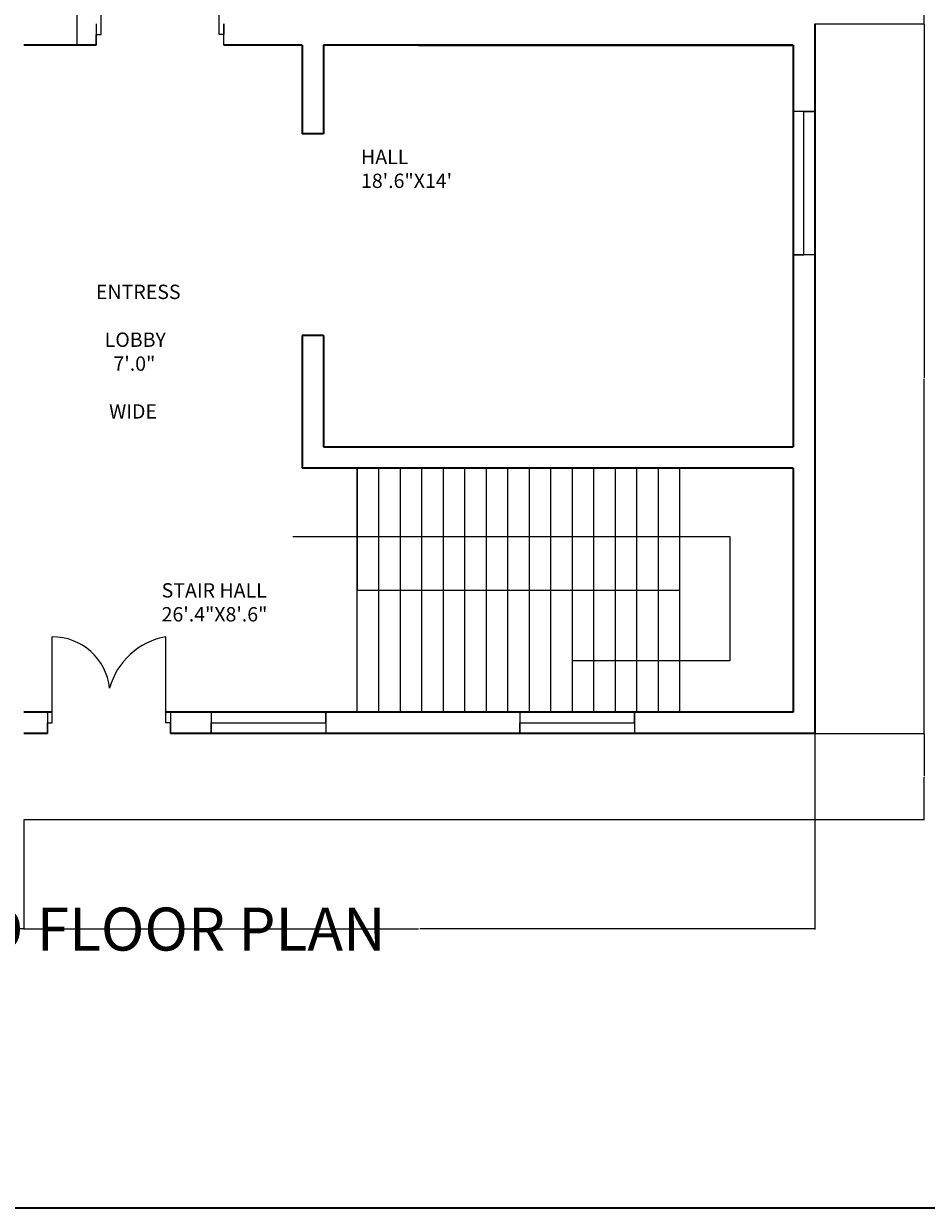
# Model space of a CAD drawing. Units: inches. Extents: x 1824 to 3509, y 619 to 2294.
# Tile 2 of 12: x 2192 to 2570, y 619 to 1115. Entities that reach past the tile are written whole.
import ezdxf

# ---------------------------------------------------------------- set-up
doc = ezdxf.new("R2010")
doc.units = ezdxf.units.IN
for name, color, linetype, lineweight in [('A-ANNO-DIMS', 2, 'Continuous', 18), ('A-ANNO-TEXT', 7, 'Continuous', 25), ('A-ANNO-TTLB', 7, 'Continuous', 35), ('A-AREA-IDEN', 7, 'Continuous', 18), ('A-DOOR', 3, 'Continuous', 18), ('A-FLOR-STRS', 7, 'Continuous', 18), ('A-GLAZ', 4, 'Continuous', 18), ('A-WALL', 7, 'Continuous', 35)]:
    doc.layers.add(name, color=color, linetype=linetype, lineweight=lineweight)
doc.styles.get("Standard").update_dxf_attribs({"font": 'arial.ttf'})
doc.dimstyles.get("Standard").update_dxf_attribs({"dimtxt": 0.18, "dimasz": 0.18, "dimexe": 0.18, "dimexo": 0.0625, "dimgap": 0.09, "dimtad": 0, "dimtih": 1, "dimtoh": 1, "dimdec": 4, "dimzin": 0, "dimdsep": 46, "dimtxsty": 'Standard', "dimcen": 0.09, "dimadec": 0, "dimazin": 0, "dimtfac": 1, "dimtdec": 4, "dimtofl": 0, "dimtmove": 0, "dimatfit": 3, "dimfxl": 1, "dimtolj": 1, "dimtzin": 0, "dimarcsym": 0})

# ---------------------------------------------------------------- blocks, each defined once
blk = doc.blocks.new('STAIR-RETURN-PLAN')
for p, q in [((26.85, 0), (26.85, 102)), ((26.85, 102), (26.85, 51)), ((35.85, 102), (35.85, 0)), ((44.85, 102), (44.85, 0)), ((53.85, 102), (53.85, 0)), ((62.85, 102), (62.85, 0)), ((71.85, 102), (71.85, 0)), ((80.85, 102), (80.85, 0)), ((89.85, 102), (89.85, 0)), ((98.85, 102), (98.85, 0)), ((107.85, 102), (107.85, 0)), ((116.85, 102), (116.85, 0)), ((125.85, 102), (125.85, 0)), ((134.85, 102), (134.85, 0)), ((143.85, 102), (143.85, 0)), ((152.85, 102), (152.85, 0)), ((161.85, 102), (161.85, 0)), ((0, 73.44), (182.85, 73.44)), ((182.85, 73.44), (182.85, 21.48)), ((26.85, 51), (161.85, 51)), ((182.85, 21.48), (116.85, 21.48))]:
    blk.add_line(p, q)
blk = doc.blocks.new('DOOR-LOUNGE-PAIR')
for p, q in [((2, 4.5), (2, 40.5)), ((51.41, 4.5), (51.41, 40.5)), ((27.9, 14.63), (27.9, 18.05)), ((0, 9), (0, 0)), ((53.41, 0), (53.41, 9)), ((53.41, 9), (53.41, 4.5)), ((0, 0), (0, 4.5)), ((0, 4.5), (2, 4.5)), ((53.41, 4.5), (51.41, 4.5)), ((53.41, 4.5), (53.41, 4.5))]:
    blk.add_line(p, q)
for centre, radius, start, end in [((-0.78, 11.81), 28.82, 5.6014, 84.4566), ((54.5, 13.67), 27.01, 96.5732, 173.8895)]:
    blk.add_arc(centre, radius, start, end)
blk = doc.blocks.new('DOOR-ENTRY-PAIR')
for p, q in [((2, 4.5), (2, 40.5)), ((49.54, 4.5), (49.54, 40.5)), ((0, 9), (0, 0)), ((51.54, 9), (51.54, 0)), ((0, 0), (0, 4.5)), ((0, 4.5), (2, 4.5)), ((51.54, 4.5), (49.54, 4.5)), ((51.54, 0), (51.54, 4.5))]:
    blk.add_line(p, q)
for centre, radius, start, end in [((2, 16.28), 24.22, 6.4131, 90), ((54.84, 11.16), 29.82, 100.2425, 164.7797)]:
    blk.add_arc(centre, radius, start, end)
blk = doc.blocks.new('WIN-48')
for p, q in [((0, 9), (0, 0)), ((48, 4.5), (48, 9)), ((48, 9), (48, 0)), ((0, 0), (0, 4.5)), ((0, 4.5), (48, 4.5))]:
    blk.add_line(p, q)
blk = doc.blocks.new('WIN-60')
for p, q in [((0, 9), (0, 0)), ((60, 4.5), (60, 9)), ((60, 9), (60, 0)), ((0, 0), (0, 4.5)), ((0, 4.5), (60, 4.5))]:
    blk.add_line(p, q)
blk = doc.blocks.new('*D75')
at = {"layer": 'A-ANNO-DIMS', "color": 0, "lineweight": -2, "transparency": 16777216}
for p, q in [((2222.38, 1146.6), (2214.25, 1146.6)), ((2214.43, 1146.42), (2214.43, 1126.53)), ((2214.43, 1106.28), (2214.43, 1126.17)), ((2222.38, 1106.1), (2214.25, 1106.1))]:
    blk.add_line(p, q, dxfattribs=at)
at = {"layer": 'A-ANNO-DIMS', "color": 0, "transparency": 16777216}
for points in [[(2214.4, 1146.42), (2214.46, 1146.42), (2214.43, 1146.6)], [(2214.4, 1106.28), (2214.46, 1106.28), (2214.43, 1106.1)]]:
    blk.add_solid(points, dxfattribs=at)
at = {"layer": 'Defpoints', "color": 0, "transparency": 16777216}
for p in [(2214.43, 1146.6), (2222.44, 1146.6), (2222.44, 1106.1)]:
    blk.add_point(p, dxfattribs=at)
at = {"layer": 'A-ANNO-DIMS', "color": 0, "transparency": 16777216, "insert": (2214.43, 1126.35), "char_height": 0.18, "attachment_point": 5}
blk.add_mtext('\\A1;41 TYP.', dxfattribs=at)
blk = doc.blocks.new('*D94')
at = {"layer": 'A-ANNO-DIMS', "color": 0, "lineweight": -2, "transparency": 16777216}
for p, q in [((1949.09, 1049.16), (1949.09, 1668.03)), ((1949.27, 1667.85), (2235.8, 1667.85)), ((2522.91, 1667.85), (2236.38, 1667.85)), ((2523.09, 1622.16), (2523.09, 1668.03))]:
    blk.add_line(p, q, dxfattribs=at)
at = {"layer": 'A-ANNO-DIMS', "color": 0, "transparency": 16777216}
for points in [[(1949.27, 1667.88), (1949.27, 1667.82), (1949.09, 1667.85)], [(2522.91, 1667.88), (2522.91, 1667.82), (2523.09, 1667.85)]]:
    blk.add_solid(points, dxfattribs=at)
at = {"layer": 'Defpoints', "color": 0, "transparency": 16777216}
for p in [(2523.09, 1667.85), (2523.09, 1622.1), (1949.09, 1049.1)]:
    blk.add_point(p, dxfattribs=at)
at = {"layer": 'A-ANNO-DIMS', "color": 0, "transparency": 16777216, "insert": (2236.09, 1667.85), "char_height": 0.18, "attachment_point": 5}
blk.add_mtext('\\A1;574', dxfattribs=at)
blk = doc.blocks.new('*D96')
at = {"layer": 'A-ANNO-DIMS', "color": 0, "lineweight": -2, "transparency": 16777216}
for p, q in [((2523.15, 818.1), (2569.02, 818.1)), ((2568.84, 817.92), (2568.84, 800.28)), ((2568.84, 782.28), (2568.84, 799.92)), ((2192.15, 782.1), (2569.02, 782.1))]:
    blk.add_line(p, q, dxfattribs=at)
at = {"layer": 'A-ANNO-DIMS', "color": 0, "transparency": 16777216}
for points in [[(2568.81, 817.92), (2568.87, 817.92), (2568.84, 818.1)], [(2568.81, 782.28), (2568.87, 782.28), (2568.84, 782.1)]]:
    blk.add_solid(points, dxfattribs=at)
at = {"layer": 'Defpoints', "color": 0, "transparency": 16777216}
for p in [(2523.09, 818.1), (2568.84, 818.1), (2192.09, 782.1)]:
    blk.add_point(p, dxfattribs=at)
at = {"layer": 'A-ANNO-DIMS', "color": 0, "transparency": 16777216, "insert": (2568.84, 800.1), "char_height": 0.18, "attachment_point": 5}
blk.add_mtext('\\A1;36', dxfattribs=at)
blk = doc.blocks.new('*D97')
at = {"layer": 'A-ANNO-DIMS', "color": 0, "lineweight": -2, "transparency": 16777216}
for p, q in [((2523.15, 1115.1), (2569.02, 1115.1)), ((2568.84, 1114.92), (2568.84, 966.78)), ((2568.84, 818.28), (2568.84, 966.42)), ((2523.15, 818.1), (2569.02, 818.1))]:
    blk.add_line(p, q, dxfattribs=at)
at = {"layer": 'A-ANNO-DIMS', "color": 0, "transparency": 16777216}
for points in [[(2568.81, 1114.92), (2568.87, 1114.92), (2568.84, 1115.1)], [(2568.81, 818.28), (2568.87, 818.28), (2568.84, 818.1)]]:
    blk.add_solid(points, dxfattribs=at)
at = {"layer": 'Defpoints', "color": 0, "transparency": 16777216}
for p in [(2523.09, 1115.1), (2568.84, 1115.1), (2523.09, 818.1)]:
    blk.add_point(p, dxfattribs=at)
at = {"layer": 'A-ANNO-DIMS', "color": 0, "transparency": 16777216, "insert": (2568.84, 966.6), "char_height": 0.18, "attachment_point": 5}
blk.add_mtext('\\A1;297', dxfattribs=at)
blk = doc.blocks.new('*D98')
at = {"layer": 'A-ANNO-DIMS', "color": 0, "lineweight": -2, "transparency": 16777216}
for p, q in [((2523.15, 1235.1), (2569.02, 1235.1)), ((2568.84, 1234.92), (2568.84, 1175.28)), ((2568.84, 1115.28), (2568.84, 1174.92)), ((2523.15, 1115.1), (2569.02, 1115.1))]:
    blk.add_line(p, q, dxfattribs=at)
at = {"layer": 'A-ANNO-DIMS', "color": 0, "transparency": 16777216}
for points in [[(2568.81, 1234.92), (2568.87, 1234.92), (2568.84, 1235.1)], [(2568.81, 1115.28), (2568.87, 1115.28), (2568.84, 1115.1)]]:
    blk.add_solid(points, dxfattribs=at)
at = {"layer": 'Defpoints', "color": 0, "transparency": 16777216}
for p in [(2523.09, 1235.1), (2568.84, 1235.1), (2523.09, 1115.1)]:
    blk.add_point(p, dxfattribs=at)
at = {"layer": 'A-ANNO-DIMS', "color": 0, "transparency": 16777216, "insert": (2568.84, 1175.1), "char_height": 0.18, "attachment_point": 5}
blk.add_mtext('\\A1;120', dxfattribs=at)
blk = doc.blocks.new('*D101')
at = {"layer": 'A-ANNO-DIMS', "color": 0, "lineweight": -2, "transparency": 16777216}
for p, q in [((1949.09, 782.04), (1949.09, 736.17)), ((2192.09, 782.04), (2192.09, 736.17)), ((1949.27, 736.35), (2070.3, 736.35)), ((2191.91, 736.35), (2070.88, 736.35))]:
    blk.add_line(p, q, dxfattribs=at)
at = {"layer": 'A-ANNO-DIMS', "color": 0, "transparency": 16777216}
for points in [[(1949.27, 736.38), (1949.27, 736.32), (1949.09, 736.35)], [(2191.91, 736.38), (2191.91, 736.32), (2192.09, 736.35)]]:
    blk.add_solid(points, dxfattribs=at)
at = {"layer": 'Defpoints', "color": 0, "transparency": 16777216}
for p in [(1949.09, 782.1), (2192.09, 782.1), (2192.09, 736.35)]:
    blk.add_point(p, dxfattribs=at)
at = {"layer": 'A-ANNO-DIMS', "color": 0, "transparency": 16777216, "insert": (2070.59, 736.35), "char_height": 0.18, "attachment_point": 5}
blk.add_mtext('\\A1;243', dxfattribs=at)
blk = doc.blocks.new('*D102')
at = {"layer": 'A-ANNO-DIMS', "color": 0, "lineweight": -2, "transparency": 16777216}
for p, q in [((2523.09, 818.04), (2523.09, 736.17)), ((2192.09, 782.04), (2192.09, 736.17)), ((2192.27, 736.35), (2357.32, 736.35)), ((2522.91, 736.35), (2357.86, 736.35))]:
    blk.add_line(p, q, dxfattribs=at)
at = {"layer": 'A-ANNO-DIMS', "color": 0, "transparency": 16777216}
for points in [[(2192.27, 736.38), (2192.27, 736.32), (2192.09, 736.35)], [(2522.91, 736.38), (2522.91, 736.32), (2523.09, 736.35)]]:
    blk.add_solid(points, dxfattribs=at)
at = {"layer": 'Defpoints', "color": 0, "transparency": 16777216}
for p in [(2523.09, 818.1), (2192.09, 782.1), (2523.09, 736.35)]:
    blk.add_point(p, dxfattribs=at)
at = {"layer": 'A-ANNO-DIMS', "color": 0, "transparency": 16777216, "insert": (2357.59, 736.35), "char_height": 0.18, "attachment_point": 5}
blk.add_mtext('\\A1;331', dxfattribs=at)

msp = doc.modelspace()

# ---------------------------------------------------------------- linework, layer by layer
at = {"layer": 'A-ANNO-TTLB'}
msp.add_lwpolyline([(1824.0608, 2293.6614), (3509.3484, 2293.6614), (3509.3484, 619.4665), (1824.0608, 619.4665)], close=True, dxfattribs=at)
at = {"layer": 'A-GLAZ'}
msp.add_line((2399.6578, 827.1012), (2399.6578, 827.1012), dxfattribs=at)
at = {"layer": 'A-WALL'}
for p, q in [((2523.0899, 1115.1012), (2523.0899, 818.1012)), ((2222.4401, 1106.1012), (2192.0899, 1106.1012)), ((2308.5899, 1106.1012), (2275.8478, 1106.1012)), ((2308.5899, 1106.1012), (2308.5899, 1069.0655)), ((2514.0899, 1106.1012), (2317.5899, 1106.1012)), ((2317.5899, 1106.1012), (2317.5899, 1069.0655)), ((2317.5899, 1106.1012), (2317.5899, 1069.0655)), ((2357.0899, 1106.1012), (2514.0899, 1106.1012)), ((2514.0899, 1106.1012), (2514.0899, 938.1012)), ((2317.5899, 1069.0655), (2308.5899, 1069.0655)), ((2317.5899, 1069.0655), (2317.5899, 1069.0655)), ((2317.5899, 984.6189), (2308.5899, 984.6189)), ((2308.5899, 984.6189), (2308.5899, 929.1012)), ((2317.5899, 984.6189), (2317.5899, 938.1012)), ((2317.5899, 984.6189), (2317.5899, 938.1012)), ((2317.5899, 938.1012), (2514.0899, 938.1012)), ((2514.0899, 929.1012), (2308.5899, 929.1012)), ((2514.0899, 929.1012), (2514.0899, 827.1012)), ((2203.9846, 827.1012), (2192.0899, 827.1012)), ((2514.0899, 827.1012), (2251.5256, 827.1012)), ((2201.9846, 818.1012), (2192.0899, 818.1012)), ((2523.0899, 818.1012), (2253.5256, 818.1012))]:
    msp.add_line(p, q, dxfattribs=at)

# ---------------------------------------------------------------- block references
at = {"layer": 'A-DOOR'}
for name, p in [('DOOR-LOUNGE-PAIR', (2222.44, 1106.101)), ('DOOR-ENTRY-PAIR', (2201.985, 818.101))]:
    msp.add_blockref(name, p, dxfattribs=at)
at = {"layer": 'A-FLOR-STRS'}
msp.add_blockref('STAIR-RETURN-PLAN', (2304.722, 827.101), dxfattribs=at)
at = {"layer": 'A-GLAZ', "extrusion": (0, 0, -1), "zscale": -1, "rotation": 90}
msp.add_blockref('WIN-60', (-2514.0897, 1018.336), dxfattribs=at)
at = {"layer": 'A-GLAZ'}
for p in [(2270.485, 818.101), (2399.658, 818.101)]:
    msp.add_blockref('WIN-48', p, dxfattribs=at)

# ---------------------------------------------------------------- texts
at = {"layer": 'A-ANNO-TEXT', "insert": (2088.9129, 745.2888), "char_height": 18, "attachment_point": 1}
msp.add_mtext_dynamic_manual_height_columns('GROUND FLOOR PLAN', width=638.440451, gutter_width=12.5, heights=[0], dxfattribs=at)
at = {"layer": 'A-AREA-IDEN', "char_height": 6, "attachment_point": 1}
for s, width, insert in [('HALL\\P18\'.6"X14\'', 156.047439, (2333.2319, 1062.3706)), ('ENTRESS\\P\\P  LOBBY\\P  \\P    7\'.0"\\P\\P   WIDE', 139.671109, (2222.3201, 1005.8947)), ('STAIR HALL\\P26\'.4"X8\'.6"', 77.837365, (2249.7956, 881.0034))]:
    msp.add_mtext_dynamic_manual_height_columns(s, width=width, gutter_width=12.5, heights=[0], dxfattribs=dict(at, insert=insert))

# ---------------------------------------------------------------- dimensions: what is measured, and where the dimension line sits
at = {"layer": 'A-ANNO-DIMS'}
for base, p1, p2, picture, middle in [((2523.0899, 1667.8512), (1949.0899, 1049.1012), (2523.0899, 1622.1012), '*D94', (2236.0899, 1667.8512)), ((2523.0899, 736.3512), (2192.0899, 782.1012), (2523.0899, 818.1012), '*D102', (2357.5899, 736.3512)), ((2192.0899, 736.3512), (1949.0899, 782.1012), (2192.0899, 782.1012), '*D101', (2070.5899, 736.3512))]:
    dim = msp.add_linear_dim(base=base, p1=p1, p2=p2, dimstyle='Standard', override={"dimdec": 0, "dimlfac": 1, "dimrnd": 0, "dimzin": 0, "dimdsep": 46, "dimlunit": 2}, dxfattribs=at)
    dim.commit()
    dim.dimension.update_dxf_attribs({"geometry": picture, "text_midpoint": middle})
for base, p1, p2, picture, middle in [((2568.8399, 1235.1012), (2523.0899, 1115.1012), (2523.0899, 1235.1012), '*D98', (2568.8399, 1175.1012)), ((2568.8399, 1115.1012), (2523.0899, 818.1012), (2523.0899, 1115.1012), '*D97', (2568.8399, 966.6012)), ((2568.8399, 818.1012), (2192.0899, 782.1012), (2523.0899, 818.1012), '*D96', (2568.8399, 800.1012))]:
    dim = msp.add_linear_dim(base=base, p1=p1, p2=p2, angle=90, dimstyle='Standard', override={"dimdec": 0, "dimlfac": 1, "dimrnd": 0, "dimzin": 0, "dimdsep": 46, "dimlunit": 2}, dxfattribs=at)
    dim.commit()
    dim.dimension.update_dxf_attribs({"geometry": picture, "text_midpoint": middle})
dim = msp.add_linear_dim(base=(2214.4289424785, 1146.6011662656), p1=(2222.4400938008, 1106.1011662656), p2=(2222.4400938008, 1146.6011662656), angle=90, text='<> TYP.', dimstyle='Standard', override={"dimdec": 0, "dimlfac": 1, "dimrnd": 0, "dimzin": 0, "dimdsep": 46, "dimlunit": 2}, dxfattribs=at)
dim.commit()
dim.dimension.update_dxf_attribs({"geometry": '*D75', "text_midpoint": (2214.4289424785, 1126.3511662656)})

doc.saveas('drawing.dxf')
